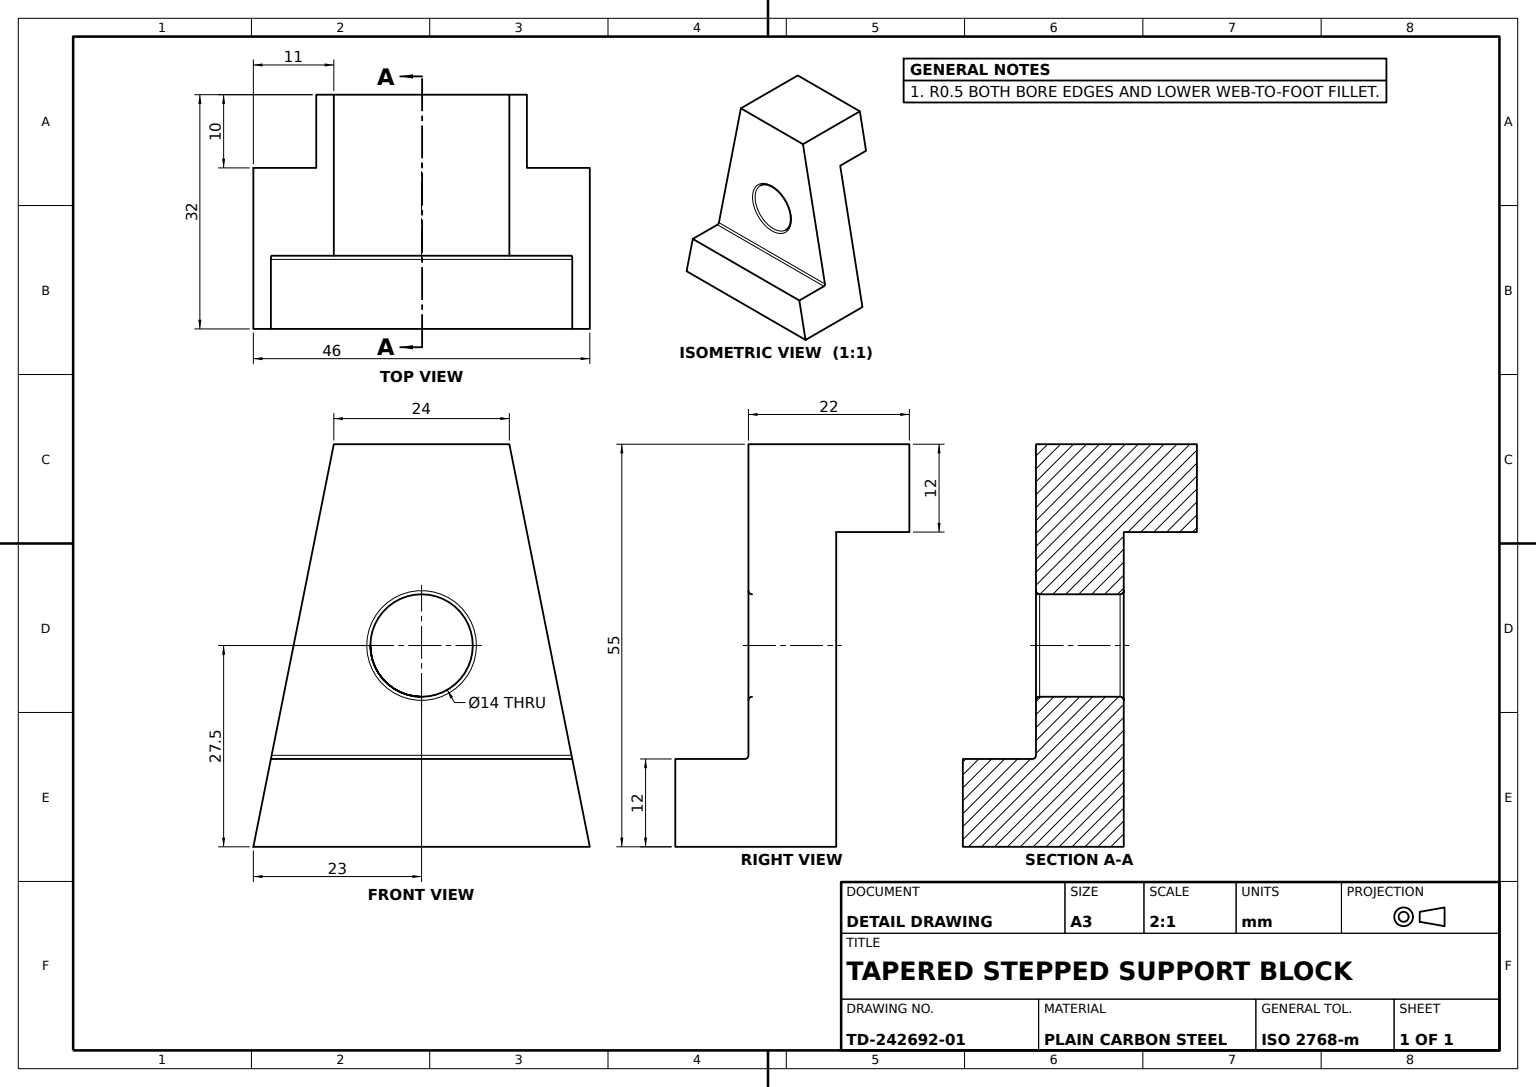
from build123d import *

# Parameters (mm, degrees)
BRACKET_BODY_DEPTH        = 46
TAPERED_SIDE_CUT_DEPTH    = 46
BORE_SKETCH_R             = 7
THROUGH_BORE_14_DEPTH     = 46
BORE_EDGE_FILLET_R0_5_A_R = 0.5
BORE_EDGE_FILLET_R0_5_B_R = 0.5
STEP_EDGE_FILLET_R0_5_R   = 0.5


with BuildPart() as part:
    # Bracket Profile Sketch → Bracket Body (new body)
    with BuildSketch(Plane.XY):
        Polygon((0, 0), (22, 0), (22, 12), (12, 12), (12, 55), (-10, 55), (-10, 43), (0, 43), align=None)
    extrude(amount=BRACKET_BODY_DEPTH)

    # Taper Cut Sketch → Tapered Side Cut (cut)
    with BuildSketch(Plane(origin=(22, 0, 0), x_dir=(0, 0, -1), z_dir=(1, 0, 0))):
        Polygon((-46, 0), (-35, 55), (-46, 55), align=None)
        Polygon((0, 0), (0, 55), (-11, 55), align=None)
    extrude(amount=-TAPERED_SIDE_CUT_DEPTH, mode=Mode.SUBTRACT)

    # Bore Sketch → Through Bore Ø14 (cut)
    with BuildSketch(Plane.ZY):
        with Locations(Location((23, 27.5, 0), (0, 0, 270))):
            Circle(BORE_SKETCH_R)
    extrude(amount=-THROUGH_BORE_14_DEPTH, mode=Mode.SUBTRACT)

    # Bore Edge Fillet R0.5 A
    bore_edge_fillet_r0_5_a_edges = [part.edges().sort_by_distance(p)[0] for p in [
        (12, 34.5, 23),
    ]]
    fillet(bore_edge_fillet_r0_5_a_edges, radius=BORE_EDGE_FILLET_R0_5_A_R)

    # Bore Edge Fillet R0.5 B
    bore_edge_fillet_r0_5_b_edges = [part.edges().sort_by_distance(p)[0] for p in [
        (0, 34.5, 23),
    ]]
    fillet(bore_edge_fillet_r0_5_b_edges, radius=BORE_EDGE_FILLET_R0_5_B_R)

    # Step Edge Fillet R0.5
    step_edge_fillet_r0_5_edges = [part.edges().sort_by_distance(p)[0] for p in [
        (12, 12, 23),
    ]]
    fillet(step_edge_fillet_r0_5_edges, radius=STEP_EDGE_FILLET_R0_5_R)


solid = part.part
